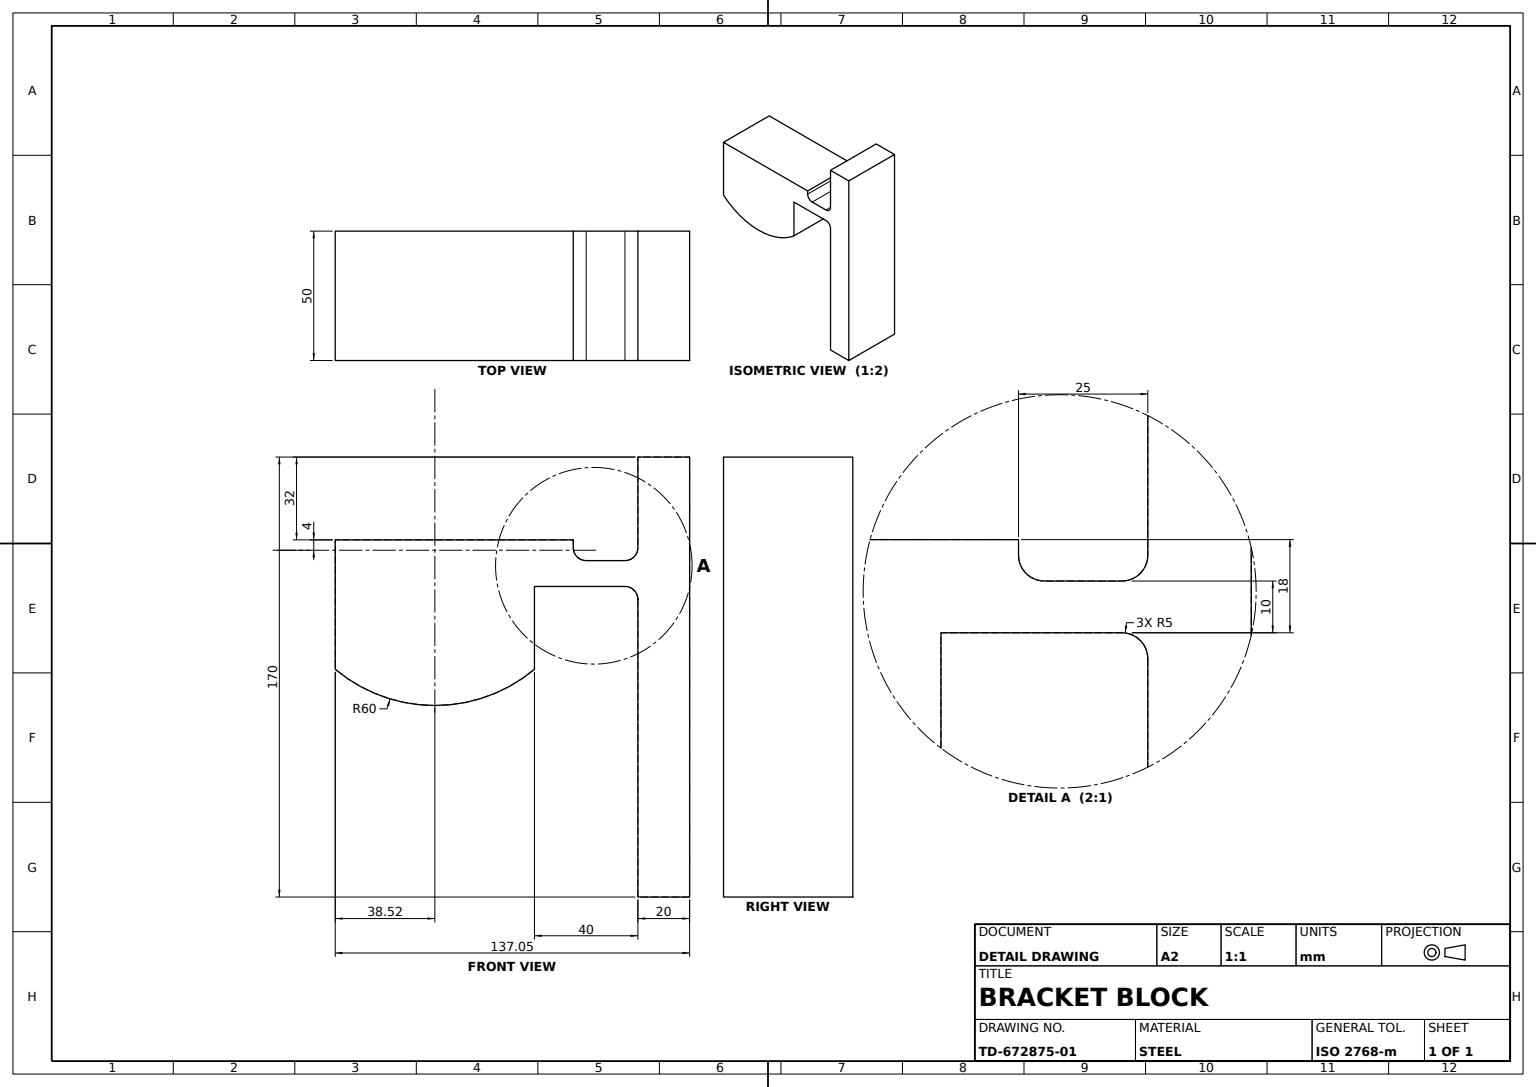
from build123d import *

# Parameters (mm, degrees)
BACK_PLATE_SKETCH_W = 20
BACK_PLATE_SKETCH_H = 170
BACK_PLATE_DEPTH    = 25
NECK_BOSS_DEPTH     = 50
NECK_FILLET_R5_R    = 5
ARM_BLOCK_DEPTH     = 50


with BuildPart() as part:
    # Back Plate Sketch → Back Plate (new, symmetric)
    with BuildSketch(Plane(origin=(0, 0, 0), x_dir=(0, 0, -1), z_dir=(1, 0, 0))):
        Rectangle(BACK_PLATE_SKETCH_W, BACK_PLATE_SKETCH_H)
    extrude(amount=BACK_PLATE_DEPTH, both=True)

    # Neck Boss Sketch → Neck Boss (add, through all)
    with BuildSketch(Plane(origin=(25, 0, 0), x_dir=(0, 0, -1), z_dir=(1, 0, 0))):
        with BuildLine():
            Line((-30, 45), (-10, 45))
            Line((-10, 45), (-10, 35))
            Line((-10, 35), (-50, 35))
            Line((-50, 35), (-50, 53))
            Line((-50, 53), (-35, 53))
            Line((-35, 53), (-35, 50))
            ThreePointArc((-35, 50), (-33.535533906, 46.464466094), (-30, 45))
        make_face()
    extrude(amount=-NECK_BOSS_DEPTH)

    # Neck Fillet R5
    neck_fillet_r5_edges = [part.edges().sort_by_distance(p)[0] for p in [
        (0, 45, 10),
        (0, 35, 10),
    ]]
    fillet(neck_fillet_r5_edges, radius=NECK_FILLET_R5_R)

    # Arm Block Sketch → Arm Block (add, through all)
    with BuildSketch(Plane(origin=(25, 0, 0), x_dir=(0, 0, -1), z_dir=(1, 0, 0))):
        with BuildLine():
            Line((-50, 53), (-50, 3))
            ThreePointArc((-50, 3), (-88.522720569, -11), (-127.045441137, 3))
            Line((-127.045441137, 3), (-127.045441137, 53))
            Line((-127.045441137, 53), (-50, 53))
        make_face()
    extrude(amount=-ARM_BLOCK_DEPTH)


solid = part.part
